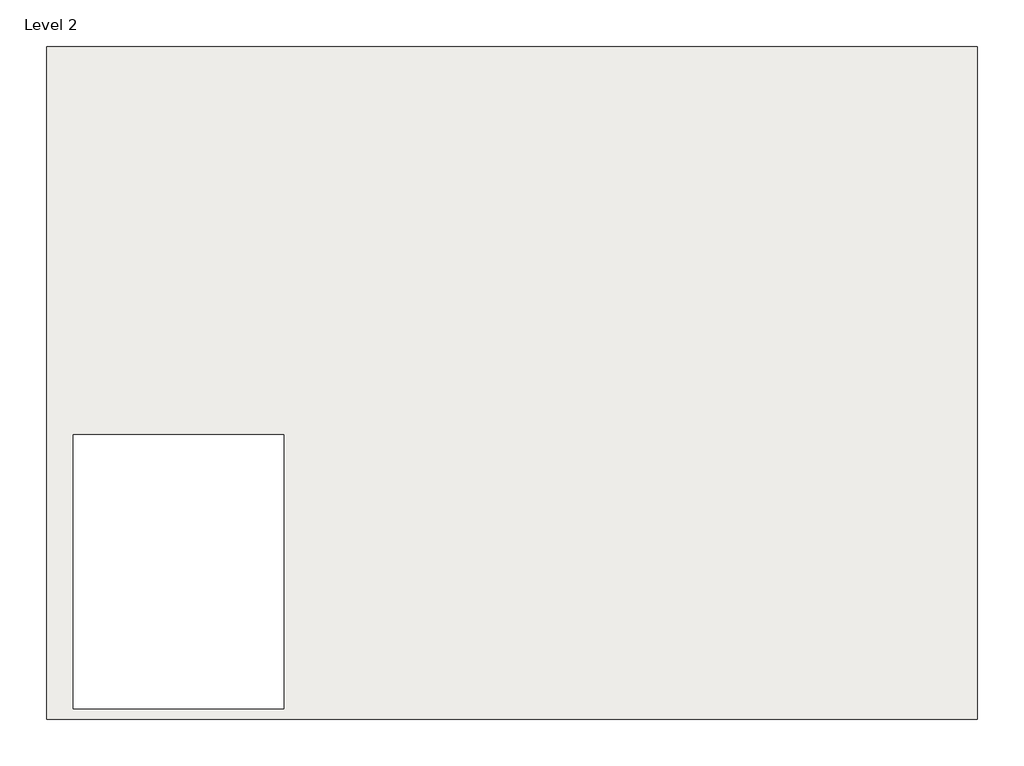
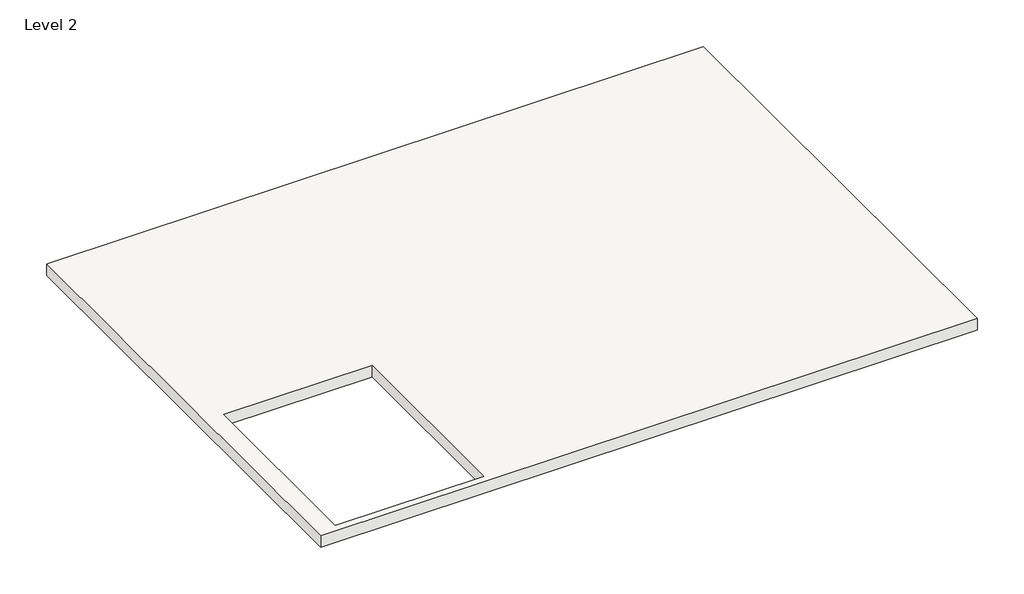
# One storey: 1 slab.
"""IFC4 building model written with IfcOpenShell, lengths in millimetres."""

from ifc_helpers import new_model, si_unit, frame, origin, place, context, project, spatial, polyline, outline, extrude, element, save

model = new_model("IFC4")

# Units and contexts
model_context = context("Model", 3, world=origin())
ifc_project = project(units=[si_unit("LENGTHUNIT", "METRE", prefix="MILLI")], contexts=[model_context])

# Site, building, storey
site = spatial("IfcSite", under=ifc_project)
building = spatial("IfcBuilding", under=site)
storey = spatial("IfcBuildingStorey", under=building, Name="Level 2", Elevation=3048.0)

# Slab
placement = place(None, origin())
element("IfcSlab", 1, ObjectType="Generic - 12\" 4", at=placement, inside=storey, context=model_context, shape_type="SweptSolid", body=[
    extrude(outline(polyline([(5525.3713479, 9866.4565451), (5525.3713479, -2057.3592285), (-10970.8984786, -2057.3592285), (-10970.8984786, 9866.4565451), (5525.3713479, 9866.4565451)]), holes=[polyline([(-6768.2286521, 2983.405876), (-10495.8098132, 2983.405876), (-10495.8098132, -1868.3434549), (-6768.2286521, -1868.3434549), (-6768.2286521, 2983.405876)])]), frame((0.0, 0.0, 3048.0), z_axis=(0.0, 0.0, 1.0), x_axis=(1.0, 0.0, 0.0)), (0.0, 0.0, 1.0), 304.8),
])

save(model, "model.ifc")

# Revit data of these elements
# Type "Generic - 12\" 4"
#   Assembly Code = "B1010"
#   Function = 0
#   Layers, outside or top first: 1' - 0" "Laminate, Ivory, Matte" (function 1)
# Element 1 (IfcSlab, "Generic - 12\" 4")
#   Height Offset From Level = 1' - 0"
#   Phase Created = New Construction
#   Materials on its faces: "Laminate, Ivory, Matte"
# Materials
#   "Laminate, Ivory, Matte": class "Plastic", colour RGB 247 247 239, transparency 0, Description = "Plastic Laminate - Ivory, Matte", Cost = 0
